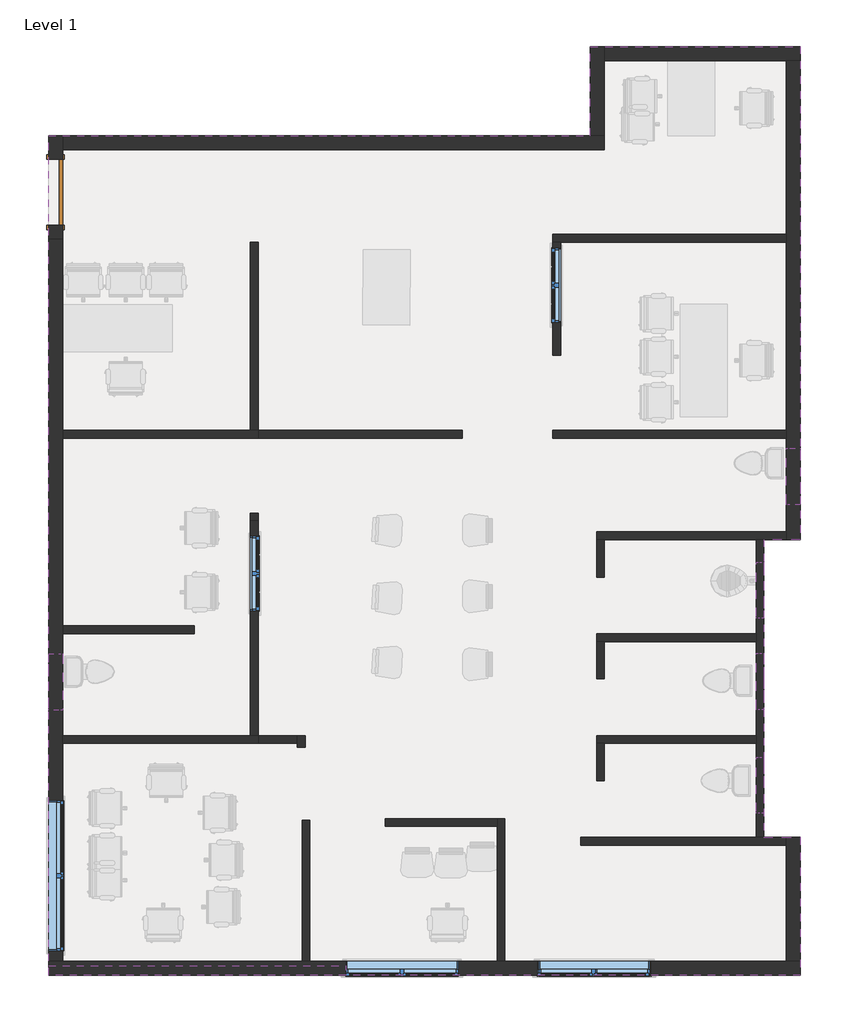
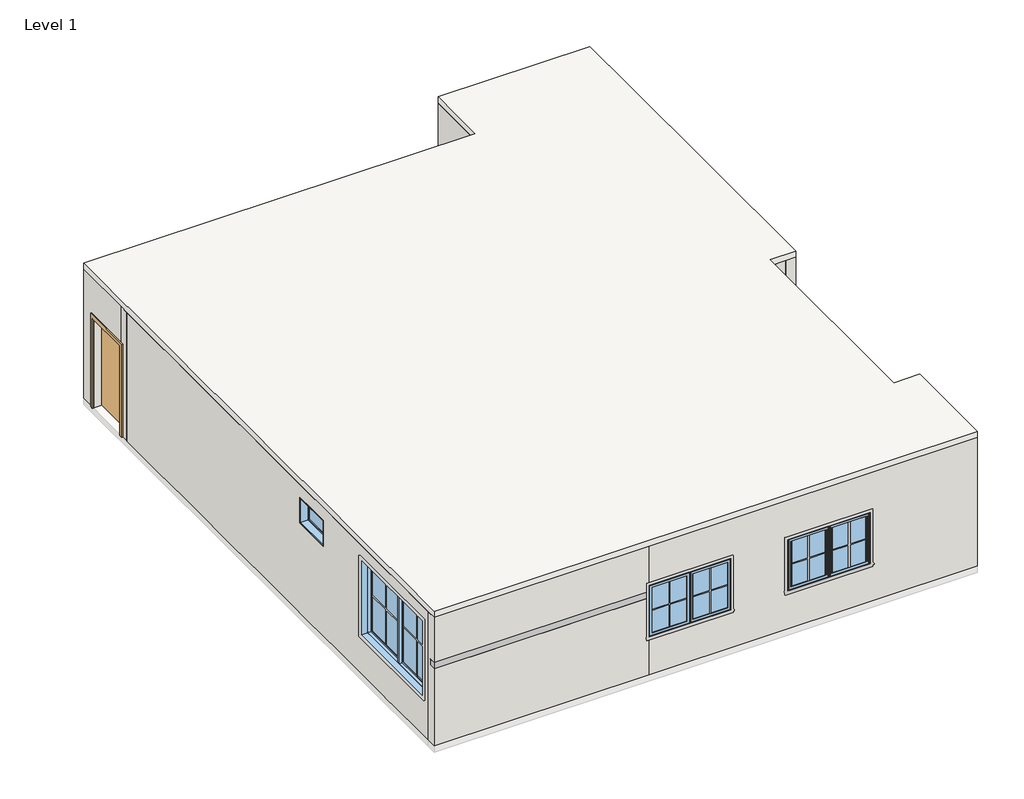
# One storey, part 1 of 2: 34 walls, 12 windows, 1 door, 1 proxy, 1 slab.
"""IFC4 building model written with IfcOpenShell, lengths in millimetres."""

from ifc_helpers import new_model, si_unit, frame, origin, origin_with_axes, place, context, project, spatial, polyline, outline, extrude, faceted_brep, transform, mapped, element, save
from components import door_0848dd25, window_12349545, window_a7c9e031, window_c8489cfa, window_casement_double_4_52a76413, window_casement_double_4_x4_bf2f09a8, window_casement_double_6_x4_44178710, window_casement_double_8_9ae172a2

model = new_model("IFC4")

# Units and contexts
model_context = context("Model", 3, world=origin())
ifc_project = project(units=[si_unit("LENGTHUNIT", "METRE", prefix="MILLI")], contexts=[model_context])

# Site, building, storey
site = spatial("IfcSite", under=ifc_project)
building = spatial("IfcBuilding", under=site)
storey = spatial("IfcBuildingStorey", under=building, Name="Level 1", Elevation=0.0)

# Proxy
placement = place(None, origin())
element("IfcBuildingElementProxy", 1, Name="Reveal", ObjectType="Reveal", at=placement, inside=storey, context=model_context, shape_type="SweptSolid", body=[
    extrude(outline(polyline([(-7315.2, -5486.4), (-7315.2, -5334.0), (-2495.8695713, -5334.0), (-2495.8695713, -5486.4), (-7315.2, -5486.4)])), frame((0.0, 0.0, 1828.8), z_axis=(0.0, 0.0, 1.0), x_axis=(1.0, 0.0, 0.0)), (0.0, 0.0, 1.0), 152.4),
])

# Door
door_shape = door_0848dd25(model_context)
element("IfcDoor", 2, ObjectType="Single-Flush : 3'6\"X7'", at=placement, inside=storey, context=model_context, shape_type="MappedRepresentation", body=[
    mapped(door_shape, transform((-7200.9, 7213.6129621, 0.0), x_axis=(0.0, 1.0, 0.0), y_axis=(-1.0, 0.0, 0.0), z_axis=(0.0, 0.0, 1.0))),
])

# Slab
element("IfcSlab", 3, ObjectType="Generic - 6\"", at=placement, inside=storey, context=model_context, shape_type="SweptSolid", body=[
    extrude(outline(polyline([(1473.2, 8128.0), (1473.2, 9575.8), (4876.8, 9575.8), (4876.8, 8128.0), (4876.8, 1574.8), (4289.425, 1574.8), (4289.425, -3251.2), (4876.8, -3251.2), (4876.8, -5486.4), (-7315.2, -5486.4), (-7315.2, 8128.0), (1473.2, 8128.0)])), frame((0.0, 0.0, 3048.0), z_axis=(0.0, 0.0, 1.0), x_axis=(1.0, 0.0, 0.0)), (0.0, 0.0, 1.0), 152.4),
])

# Walls
element("IfcWall", 4, at=placement, inside=storey, context=model_context, shape_type="Brep", body=[
    faceted_brep([(-7315.2, -5486.4, 0.0), (-2495.8695713, -5486.4, 0.0), (-2495.8695713, -5486.4, 914.4), (-2495.8695713, -5486.4, 1828.8), (-7315.2, -5486.4, 1828.8), (-2495.8695713, -5486.4, 3048.0), (-7315.2, -5486.4, 3048.0), (-7315.2, -5486.4, 1981.2), (-2495.8695713, -5486.4, 1981.2), (-2495.8695713, -5486.4, 2133.6), (-2495.8695713, -5257.8, 0.0), (-3073.4, -5257.8, 0.0), (-3200.4, -5257.8, 0.0), (-7086.6, -5257.8, 0.0), (-7315.2, -5257.8, 0.0), (-7315.2, -5257.8, 3048.0), (-7086.6, -5257.8, 3048.0), (-3200.4, -5257.8, 3048.0), (-3073.4, -5257.8, 3048.0), (-2495.8695713, -5257.8, 3048.0), (-2495.8695713, -5257.8, 2133.6), (-2495.8695713, -5257.8, 914.4), (-2495.8695713, -5334.0, 1981.2), (-2495.8695713, -5334.0, 1828.8), (-7315.2, -5334.0, 1828.8), (-7315.2, -5334.0, 1981.2)], [[[0, 1, 2, 3, 4]], [[5, 6, 7, 8, 9]], [[10, 11, 12, 13, 14, 15, 16, 17, 18, 19, 20, 21]], [[1, 0, 14, 13, 12, 11, 10]], [[10, 21, 20, 19, 5, 9, 8, 22, 23, 3, 2, 1]], [[6, 5, 19, 18, 17, 16, 15]], [[6, 15, 14, 0, 4, 24, 25, 7]], [[25, 22, 8, 7]], [[22, 25, 24, 23]], [[23, 24, 4, 3]]]),
])
element("IfcWall", 5, at=placement, inside=storey, context=model_context, shape_type="SweptSolid", body=[
    extrude(outline(polyline([(-3073.4, -2971.8), (-3073.4, -5257.8), (-3200.4, -5257.8), (-3200.4, -2971.8), (-3073.4, -2971.8)])), origin_with_axes(), (0.0, 0.0, 1.0), 3048.0),
])
element("IfcWall", 6, at=placement, inside=storey, context=model_context, shape_type="SweptSolid", body=[
    extrude(outline(polyline([(-4953.0, 50.8), (-7086.6, 50.8), (-7086.6, 177.8), (-4953.0, 177.8), (-4953.0, 50.8)])), origin_with_axes(), (0.0, 0.0, 1.0), 3048.0),
])
element("IfcWall", 7, ObjectType="3'", at=placement, inside=storey, context=model_context, shape_type="Brep", body=[
    faceted_brep([(4289.425, -3251.2, 0.0), (4289.425, 1574.8, 0.0), (4289.425, 1574.8, 3048.0), (4289.425, -3251.2, 3048.0), (4289.425, -2864.0421459, 2743.2), (4289.425, -1949.6421459, 2743.2), (4289.425, -1949.6421459, 2133.6), (4289.425, -2864.0421459, 2133.6), (4289.425, -266.6798193, 2743.2), (4289.425, -266.6798193, 2133.6), (4289.425, -1181.0798193, 2133.6), (4289.425, -1181.0798193, 2743.2), (4289.425, 299.1205911, 2743.2), (4289.425, 1213.5205911, 2743.2), (4289.425, 1213.5205911, 2133.6), (4289.425, 299.1205911, 2133.6), (4162.425, -3251.2, 0.0), (4162.425, -3251.2, 3048.0), (4162.425, -1727.2, 3048.0), (4162.425, -1600.2, 3048.0), (4162.425, -76.2, 3048.0), (4162.425, 50.8, 3048.0), (4162.425, 1574.8, 3048.0), (4162.425, 1574.8, 0.0), (4162.425, 50.8, 0.0), (4162.425, -76.2, 0.0), (4162.425, -1600.2, 0.0), (4162.425, -1727.2, 0.0), (4162.425, -2864.0421459, 2743.2), (4162.425, -2864.0421459, 2133.6), (4162.425, -1949.6421459, 2133.6), (4162.425, -1949.6421459, 2743.2), (4162.425, -266.6798193, 2743.2), (4162.425, -1181.0798193, 2743.2), (4162.425, -1181.0798193, 2133.6), (4162.425, -266.6798193, 2133.6), (4162.425, 299.1205911, 2743.2), (4162.425, 299.1205911, 2133.6), (4162.425, 1213.5205911, 2133.6), (4162.425, 1213.5205911, 2743.2)], [[[0, 1, 2, 3], [4, 5, 6, 7], [8, 9, 10, 11], [12, 13, 14, 15]], [[16, 17, 18, 19, 20, 21, 22, 23, 24, 25, 26, 27], [28, 29, 30, 31], [32, 33, 34, 35], [36, 37, 38, 39]], [[1, 0, 16, 27, 26, 25, 24, 23]], [[3, 2, 22, 21, 20, 19, 18, 17]], [[0, 3, 17, 16]], [[2, 1, 23, 22]], [[29, 28, 4, 7]], [[30, 29, 7, 6]], [[31, 30, 6, 5]], [[28, 31, 5, 4]], [[9, 8, 32, 35]], [[10, 9, 35, 34]], [[11, 10, 34, 33]], [[8, 11, 33, 32]], [[37, 36, 12, 15]], [[38, 37, 15, 14]], [[39, 38, 14, 13]], [[36, 39, 13, 12]]]),
])
element("IfcWall", 8, ObjectType="WALL11", at=placement, inside=storey, context=model_context, shape_type="Brep", body=[
    faceted_brep([(-2495.8695713, -5486.4, 0.0), (4876.8, -5486.4, 0.0), (4876.8, -5486.4, 3048.0), (-2495.8695713, -5486.4, 3048.0), (-2495.8695713, -5486.4, 2133.6), (-667.0695713, -5486.4, 2133.6), (-667.0695713, -5486.4, 914.4), (-2495.8695713, -5486.4, 914.4), (2463.8, -5486.4, 914.4), (609.6, -5486.4, 914.4), (609.6, -5486.4, 2133.6), (2463.8, -5486.4, 2133.6), (4876.8, -5257.8, 0.0), (4648.2, -5257.8, 0.0), (88.9, -5257.8, 0.0), (-38.1, -5257.8, 0.0), (-2495.8695713, -5257.8, 0.0), (-2495.8695713, -5257.8, 914.4), (-667.0695713, -5257.8, 914.4), (-667.0695713, -5257.8, 2133.6), (-2495.8695713, -5257.8, 2133.6), (-2495.8695713, -5257.8, 3048.0), (-38.1, -5257.8, 3048.0), (88.9, -5257.8, 3048.0), (4648.2, -5257.8, 3048.0), (4876.8, -5257.8, 3048.0), (2463.8, -5257.8, 2133.6), (609.6, -5257.8, 2133.6), (609.6, -5257.8, 914.4), (2463.8, -5257.8, 914.4)], [[[0, 1, 2, 3, 4, 5, 6, 7], [8, 9, 10, 11]], [[12, 13, 14, 15, 16, 17, 18, 19, 20, 21, 22, 23, 24, 25], [26, 27, 28, 29]], [[1, 0, 16, 15, 14, 13, 12]], [[3, 2, 25, 24, 23, 22, 21]], [[3, 21, 20, 4]], [[16, 0, 7, 17]], [[2, 1, 12, 25]], [[5, 19, 18, 6]], [[6, 18, 17, 7]], [[19, 5, 4, 20]], [[28, 27, 10, 9]], [[28, 9, 8, 29]], [[10, 27, 26, 11]], [[29, 8, 11, 26]]]),
])
element("IfcWall", 9, ObjectType="WALL12", at=placement, inside=storey, context=model_context, shape_type="Brep", body=[
    faceted_brep([(4876.8, -5257.8, 0.0), (4876.8, -3251.2, 0.0), (4876.8, -3251.2, 3048.0), (4876.8, -5257.8, 3048.0), (4648.2, -5257.8, 0.0), (4648.2, -5257.8, 3048.0), (4648.2, -3378.2, 3048.0), (4648.2, -3251.2, 3048.0), (4648.2, -3251.2, 0.0), (4648.2, -3378.2, 0.0)], [[[0, 1, 2, 3]], [[4, 5, 6, 7, 8, 9]], [[1, 0, 4, 9, 8]], [[3, 2, 7, 6, 5]], [[0, 3, 5, 4]], [[2, 1, 8, 7]]]),
])
element("IfcWall", 10, ObjectType="WALL13", at=placement, inside=storey, context=model_context, shape_type="Brep", body=[
    faceted_brep([(4648.2, -3251.2, 0.0), (4289.425, -3251.2, 0.0), (4162.425, -3251.2, 0.0), (1320.7323113, -3251.2, 0.0), (1320.7323113, -3251.2, 3048.0), (4162.425, -3251.2, 3048.0), (4289.425, -3251.2, 3048.0), (4648.2, -3251.2, 3048.0), (4648.2, -3378.2, 0.0), (4648.2, -3378.2, 3048.0), (1320.7323113, -3378.2, 3048.0), (1320.7323113, -3378.2, 0.0)], [[[0, 1, 2, 3, 4, 5, 6, 7]], [[8, 9, 10, 11]], [[3, 2, 1, 0, 8, 11]], [[4, 3, 11, 10]], [[7, 6, 5, 4, 10, 9]], [[0, 7, 9, 8]]]),
])
element("IfcWall", 11, ObjectType="WALL16 2", at=placement, inside=storey, context=model_context, shape_type="Brep", body=[
    faceted_brep([(4162.425, -1600.2, 0.0), (1574.8, -1600.2, 0.0), (1574.8, -1600.2, 3048.0), (4162.425, -1600.2, 3048.0), (4162.425, -1727.2, 0.0), (4162.425, -1727.2, 3048.0), (1701.8, -1727.2, 3048.0), (1574.8, -1727.2, 3048.0), (1574.8, -1727.2, 0.0), (1701.8, -1727.2, 0.0)], [[[0, 1, 2, 3]], [[4, 5, 6, 7, 8, 9]], [[1, 0, 4, 9, 8]], [[3, 2, 7, 6, 5]], [[0, 3, 5, 4]], [[2, 1, 8, 7]]]),
])
element("IfcWall", 12, ObjectType="WALL16 2", at=placement, inside=storey, context=model_context, shape_type="SweptSolid", body=[
    extrude(outline(polyline([(1574.8, -2333.2020056), (1574.8, -1727.2), (1701.8, -1727.2), (1701.8, -2333.2020056), (1574.8, -2333.2020056)])), origin_with_axes(), (0.0, 0.0, 1.0), 3048.0),
])
element("IfcWall", 13, ObjectType="WALL17", at=placement, inside=storey, context=model_context, shape_type="Brep", body=[
    faceted_brep([(4162.425, 50.8, 0.0), (1574.8, 50.8, 0.0), (1574.8, 50.8, 3048.0), (4162.425, 50.8, 3048.0), (4162.425, -76.2, 0.0), (4162.425, -76.2, 3048.0), (1701.8, -76.2, 3048.0), (1574.8, -76.2, 3048.0), (1574.8, -76.2, 0.0), (1701.8, -76.2, 0.0)], [[[0, 1, 2, 3]], [[4, 5, 6, 7, 8, 9]], [[1, 0, 4, 9, 8]], [[3, 2, 7, 6, 5]], [[0, 3, 5, 4]], [[2, 1, 8, 7]]]),
])
element("IfcWall", 14, ObjectType="WALL17", at=placement, inside=storey, context=model_context, shape_type="SweptSolid", body=[
    extrude(outline(polyline([(1574.8, -682.1332616), (1574.8, -76.2), (1701.8, -76.2), (1701.8, -682.1332616), (1574.8, -682.1332616)])), origin_with_axes(), (0.0, 0.0, 1.0), 3048.0),
])
element("IfcWall", 15, ObjectType="WALL18", at=placement, inside=storey, context=model_context, shape_type="Brep", body=[
    faceted_brep([(4648.2, 1701.8, 0.0), (1574.8, 1701.8, 0.0), (1574.8, 1701.8, 3048.0), (4648.2, 1701.8, 3048.0), (4648.2, 1574.8, 0.0), (4648.2, 1574.8, 3048.0), (4289.425, 1574.8, 3048.0), (4162.425, 1574.8, 3048.0), (1701.8, 1574.8, 3048.0), (1574.8, 1574.8, 3048.0), (1574.8, 1574.8, 0.0), (1701.8, 1574.8, 0.0), (4162.425, 1574.8, 0.0), (4289.425, 1574.8, 0.0)], [[[0, 1, 2, 3]], [[4, 5, 6, 7, 8, 9, 10, 11, 12, 13]], [[1, 0, 4, 13, 12, 11, 10]], [[3, 2, 9, 8, 7, 6, 5]], [[0, 3, 5, 4]], [[2, 1, 10, 9]]]),
])
element("IfcWall", 16, ObjectType="WALL18", at=placement, inside=storey, context=model_context, shape_type="SweptSolid", body=[
    extrude(outline(polyline([(1574.8, 965.114599), (1574.8, 1574.8), (1701.8, 1574.8), (1701.8, 965.114599), (1574.8, 965.114599)])), origin_with_axes(), (0.0, 0.0, 1.0), 3048.0),
])
element("IfcWall", 17, ObjectType="WALL19", at=placement, inside=storey, context=model_context, shape_type="SweptSolid", body=[
    extrude(outline(polyline([(863.6, 3352.8), (4648.2, 3352.8), (4648.2, 3225.8), (863.6, 3225.8), (863.6, 3352.8)])), origin_with_axes(), (0.0, 0.0, 1.0), 3048.0),
])
element("IfcWall", 18, ObjectType="WALL20", at=placement, inside=storey, context=model_context, shape_type="Brep", body=[
    faceted_brep([(4648.2, 6527.8, 0.0), (863.6, 6527.8, 0.0), (863.6, 6527.8, 3048.0), (4648.2, 6527.8, 3048.0), (4648.2, 6400.8, 0.0), (4648.2, 6400.8, 3048.0), (990.6, 6400.8, 3048.0), (863.6, 6400.8, 3048.0), (863.6, 6400.8, 0.0), (990.6, 6400.8, 0.0)], [[[0, 1, 2, 3]], [[4, 5, 6, 7, 8, 9]], [[1, 0, 4, 9, 8]], [[3, 2, 7, 6, 5]], [[0, 3, 5, 4]], [[2, 1, 8, 7]]]),
])
element("IfcWall", 19, ObjectType="WALL20", at=placement, inside=storey, context=model_context, shape_type="SweptSolid", body=[
    extrude(outline(polyline([(6400.8, 0.0), (4571.3294041, 0.0), (4571.3294041, 3048.0), (6400.8, 3048.0), (6400.8, 0.0)]), holes=[polyline([(6311.9, 2743.2), (5092.7, 2743.2), (5092.7, 914.4), (6311.9, 914.4), (6311.9, 2743.2)])]), frame((863.6, 0.0, 0.0), z_axis=(1.0, 0.0, 0.0), x_axis=(0.0, 1.0, 0.0)), (0.0, 0.0, 1.0), 127.0),
])
element("IfcWall", 20, ObjectType="WALL21", at=placement, inside=storey, context=model_context, shape_type="Brep", body=[
    faceted_brep([(-7086.6, 3225.8, 0.0), (-3911.6, 3225.8, 0.0), (-3911.6, 3225.8, 3048.0), (-7086.6, 3225.8, 3048.0), (-7086.6, 3352.8, 0.0), (-7086.6, 3352.8, 3048.0), (-4038.6, 3352.8, 3048.0), (-3911.6, 3352.8, 3048.0), (-3911.6, 3352.8, 0.0), (-4038.6, 3352.8, 0.0)], [[[0, 1, 2, 3]], [[4, 5, 6, 7, 8, 9]], [[1, 0, 4, 9, 8]], [[3, 2, 7, 6, 5]], [[0, 3, 5, 4]], [[2, 1, 8, 7]]]),
])
element("IfcWall", 21, ObjectType="WALL21", at=placement, inside=storey, context=model_context, shape_type="SweptSolid", body=[
    extrude(outline(polyline([(-3911.6, 6400.8), (-3911.6, 3352.8), (-4038.6, 3352.8), (-4038.6, 6400.8), (-3911.6, 6400.8)])), origin_with_axes(), (0.0, 0.0, 1.0), 3048.0),
])
element("IfcWall", 22, ObjectType="WALL23 2", at=placement, inside=storey, context=model_context, shape_type="Brep", body=[
    faceted_brep([(-7086.6, -1727.2, 0.0), (-3911.6, -1727.2, 0.0), (-3911.6, -1727.2, 3048.0), (-7086.6, -1727.2, 3048.0), (-7086.6, -1600.2, 0.0), (-7086.6, -1600.2, 3048.0), (-4038.6, -1600.2, 3048.0), (-3911.6, -1600.2, 3048.0), (-3911.6, -1600.2, 0.0), (-4038.6, -1600.2, 0.0)], [[[0, 1, 2, 3]], [[4, 5, 6, 7, 8, 9]], [[1, 0, 4, 9, 8]], [[3, 2, 7, 6, 5]], [[0, 3, 5, 4]], [[2, 1, 8, 7]]]),
])
element("IfcWall", 23, ObjectType="WALL23 2", at=placement, inside=storey, context=model_context, shape_type="SweptSolid", body=[
    extrude(outline(polyline([(-1600.2, 0.0), (-1600.2, 3048.0), (1880.1111463, 3048.0), (1880.1111463, 0.0), (-1600.2, 0.0)]), holes=[polyline([(419.6111463, 2743.2), (419.6111463, 914.4), (1638.8111463, 914.4), (1638.8111463, 2743.2), (419.6111463, 2743.2)])]), frame((-4038.6, 0.0, 0.0), z_axis=(1.0, 0.0, 0.0), x_axis=(0.0, 1.0, 0.0)), (0.0, 0.0, 1.0), 127.0),
])
element("IfcWall", 24, ObjectType="WALL23 2", at=placement, inside=storey, context=model_context, shape_type="SweptSolid", body=[
    extrude(outline(polyline([(-3911.6, 1880.1111463), (-4038.6, 1880.1111463), (-4038.6, 2007.1111463), (-3911.6, 2007.1111463), (-3911.6, 1880.1111463)])), origin_with_axes(), (0.0, 0.0, 1.0), 3048.0),
])
element("IfcWall", 25, ObjectType="WALL23 2", at=placement, inside=storey, context=model_context, shape_type="SweptSolid", body=[
    extrude(outline(polyline([(1880.1111463, 0.0), (-1600.2, 0.0), (-1600.2, 3048.0), (1880.1111463, 3048.0), (1880.1111463, 0.0)]), holes=[polyline([(419.6111463, 2743.2), (419.6111463, 914.4), (1638.8111463, 914.4), (1638.8111463, 2743.2), (419.6111463, 2743.2)])]), frame((-4038.6, 0.0, 0.0), z_axis=(1.0, 0.0, 0.0), x_axis=(0.0, 1.0, 0.0)), (0.0, 0.0, 1.0), 127.0),
])
element("IfcWall", 26, ObjectType="WALL23 2", at=placement, inside=storey, context=model_context, shape_type="Brep", body=[
    faceted_brep([(-3276.6, -1600.2, 0.0), (-3276.6, -1727.2, 0.0), (-3276.6, -1790.7, 0.0), (-3276.6, -1790.7, 3048.0), (-3276.6, -1727.2, 3048.0), (-3276.6, -1600.2, 3048.0), (-3149.6, -1600.2, 0.0), (-3149.6, -1600.2, 3048.0), (-3149.6, -1790.7, 3048.0), (-3149.6, -1790.7, 0.0)], [[[0, 1, 2, 3, 4, 5]], [[6, 7, 8, 9]], [[2, 1, 0, 6, 9]], [[3, 2, 9, 8]], [[5, 4, 3, 8, 7]], [[0, 5, 7, 6]]]),
])
element("IfcWall", 27, ObjectType="WALL24", at=placement, inside=storey, context=model_context, shape_type="SweptSolid", body=[
    extrude(outline(polyline([(-3276.6, -1727.2), (-3911.6, -1727.2), (-3911.6, -1600.2), (-3276.6, -1600.2), (-3276.6, -1727.2)])), origin_with_axes(), (0.0, 0.0, 1.0), 3048.0),
])
element("IfcWall", 28, ObjectType="WALL26", at=placement, inside=storey, context=model_context, shape_type="SweptSolid", body=[
    extrude(outline(polyline([(-601.4207418, 3225.8), (-3911.6, 3225.8), (-3911.6, 3352.8), (-601.4207418, 3352.8), (-601.4207418, 3225.8)])), origin_with_axes(), (0.0, 0.0, 1.0), 3048.0),
])
element("IfcWall", 29, ObjectType="WALL28", at=placement, inside=storey, context=model_context, shape_type="Brep", body=[
    faceted_brep([(88.9, -5257.8, 0.0), (88.9, -2946.3624245, 0.0), (88.9, -2946.3624245, 3048.0), (88.9, -5257.8, 3048.0), (-38.1, -5257.8, 0.0), (-38.1, -5257.8, 3048.0), (-38.1, -3073.3624245, 3048.0), (-38.1, -2946.3624245, 3048.0), (-38.1, -2946.3624245, 0.0), (-38.1, -3073.3624245, 0.0)], [[[0, 1, 2, 3]], [[4, 5, 6, 7, 8, 9]], [[1, 0, 4, 9, 8]], [[3, 2, 7, 6, 5]], [[0, 3, 5, 4]], [[2, 1, 8, 7]]]),
])
element("IfcWall", 30, ObjectType="WALL29", at=placement, inside=storey, context=model_context, shape_type="SweptSolid", body=[
    extrude(outline(polyline([(-1854.625458, -2946.3624245), (-38.1, -2946.3624245), (-38.1, -3073.3624245), (-1854.625458, -3073.3624245), (-1854.625458, -2946.3624245)])), origin_with_axes(), (0.0, 0.0, 1.0), 3048.0),
])
element("IfcWall", 31, ObjectType="WALL6", at=placement, inside=storey, context=model_context, shape_type="Brep", body=[
    faceted_brep([(-7086.6, 8128.0, 3048.0), (-7086.6, 7899.4, 3048.0), (-7086.6, 6680.2210262, 3048.0), (-7086.6, 6680.2210262, 2133.6), (-7086.6, 7747.0129621, 2133.6), (-7086.6, 7747.0129621, 0.0), (-7086.6, 7899.4, 0.0), (-7086.6, 8128.0, 0.0), (-7315.2, 6680.2210262, 3048.0), (-7315.2, 8128.0, 3048.0), (-7315.2, 8128.0, 0.0), (-7315.2, 7747.0129621, 0.0), (-7315.2, 7747.0129621, 2133.6), (-7315.2, 6680.2210262, 2133.6)], [[[0, 1, 2, 3, 4, 5, 6, 7]], [[8, 9, 10, 11, 12, 13]], [[10, 7, 6, 5, 11]], [[2, 1, 0, 9, 8]], [[0, 7, 10, 9]], [[2, 8, 13, 3]], [[4, 12, 11, 5]], [[12, 4, 3, 13]]]),
])
element("IfcWall", 32, ObjectType="WALL6", at=placement, inside=storey, context=model_context, shape_type="Brep", body=[
    faceted_brep([(-7086.6, 7899.4, 0.0), (1701.8, 7899.4, 0.0), (1701.8, 7899.4, 3048.0), (-7086.6, 7899.4, 3048.0), (-7086.6, 8128.0, 0.0), (-7086.6, 8128.0, 3048.0), (1473.2, 8128.0, 3048.0), (1701.8, 8128.0, 3048.0), (1701.8, 8128.0, 0.0), (1473.2, 8128.0, 0.0)], [[[0, 1, 2, 3]], [[4, 5, 6, 7, 8, 9]], [[1, 0, 4, 9, 8]], [[3, 2, 7, 6, 5]], [[0, 3, 5, 4]], [[2, 1, 8, 7]]]),
])
element("IfcWall", 33, ObjectType="WALL6", at=placement, inside=storey, context=model_context, shape_type="Brep", body=[
    faceted_brep([(1701.8, 8128.0, 0.0), (1701.8, 9347.2, 0.0), (1701.8, 9575.8, 0.0), (1701.8, 9575.8, 3048.0), (1701.8, 9347.2, 3048.0), (1701.8, 8128.0, 3048.0), (1473.2, 8128.0, 0.0), (1473.2, 8128.0, 3048.0), (1473.2, 9575.8, 3048.0), (1473.2, 9575.8, 0.0)], [[[0, 1, 2, 3, 4, 5]], [[6, 7, 8, 9]], [[2, 1, 0, 6, 9]], [[5, 4, 3, 8, 7]], [[0, 5, 7, 6]], [[3, 2, 9, 8]]]),
])
element("IfcWall", 34, ObjectType="WALL8", at=placement, inside=storey, context=model_context, shape_type="Brep", body=[
    faceted_brep([(1701.8, 9347.2, 0.0), (4648.2, 9347.2, 0.0), (4876.8, 9347.2, 0.0), (4876.8, 9347.2, 3048.0), (4648.2, 9347.2, 3048.0), (1701.8, 9347.2, 3048.0), (1701.8, 9575.8, 0.0), (1701.8, 9575.8, 3048.0), (4876.8, 9575.8, 3048.0), (4876.8, 9575.8, 0.0)], [[[0, 1, 2, 3, 4, 5]], [[6, 7, 8, 9]], [[2, 1, 0, 6, 9]], [[5, 4, 3, 8, 7]], [[0, 5, 7, 6]], [[3, 2, 9, 8]]]),
])
element("IfcWall", 35, ObjectType="WALL8", at=placement, inside=storey, context=model_context, shape_type="Brep", body=[
    faceted_brep([(4648.2, 9347.2, 0.0), (4648.2, 6527.8, 0.0), (4648.2, 6400.8, 0.0), (4648.2, 3352.8, 0.0), (4648.2, 3225.8, 0.0), (4648.2, 1701.8, 0.0), (4648.2, 1574.8, 0.0), (4648.2, 1574.8, 3048.0), (4648.2, 1701.8, 3048.0), (4648.2, 3225.8, 3048.0), (4648.2, 3352.8, 3048.0), (4648.2, 6400.8, 3048.0), (4648.2, 6527.8, 3048.0), (4648.2, 9347.2, 3048.0), (4648.2, 3060.7, 2743.2), (4648.2, 2146.3, 2743.2), (4648.2, 2146.3, 2133.6), (4648.2, 3060.7, 2133.6), (4876.8, 9347.2, 0.0), (4876.8, 9347.2, 3048.0), (4876.8, 1574.8, 3048.0), (4876.8, 1574.8, 0.0), (4876.8, 3060.7, 2743.2), (4876.8, 3060.7, 2133.6), (4876.8, 2146.3, 2133.6), (4876.8, 2146.3, 2743.2)], [[[0, 1, 2, 3, 4, 5, 6, 7, 8, 9, 10, 11, 12, 13], [14, 15, 16, 17]], [[18, 19, 20, 21], [22, 23, 24, 25]], [[6, 5, 4, 3, 2, 1, 0, 18, 21]], [[13, 12, 11, 10, 9, 8, 7, 20, 19]], [[0, 13, 19, 18]], [[7, 6, 21, 20]], [[23, 22, 14, 17]], [[24, 23, 17, 16]], [[25, 24, 16, 15]], [[22, 25, 15, 14]]]),
])
element("IfcWall", 36, ObjectType="WALL9", at=placement, inside=storey, context=model_context, shape_type="Brep", body=[
    faceted_brep([(-7315.2, 6451.6210262, 0.0), (-7086.6, 6451.6210262, 0.0), (-7086.6, 6451.6210262, 3048.0), (-7315.2, 6451.6210262, 3048.0), (-7315.2, 6680.2210262, 0.0), (-7315.2, 6680.2210262, 2133.6), (-7315.2, 6680.2210262, 3048.0), (-7086.6, 6680.2210262, 3048.0), (-7086.6, 6680.2210262, 2133.6), (-7086.6, 6680.2210262, 0.0)], [[[0, 1, 2, 3]], [[4, 5, 6, 7, 8, 9]], [[1, 0, 4, 9]], [[3, 2, 7, 6]], [[0, 3, 6, 5, 4]], [[2, 1, 9, 8, 7]]]),
])
element("IfcWall", 37, ObjectType="WALL9", at=placement, inside=storey, context=model_context, shape_type="Brep", body=[
    faceted_brep([(-7315.2, 6451.6210262, 0.0), (-7315.2, -5257.8, 0.0), (-7315.2, -5257.8, 3048.0), (-7315.2, 6451.6210262, 3048.0), (-7315.2, -273.05, 2743.2), (-7315.2, -1187.45, 2743.2), (-7315.2, -1187.45, 2133.6), (-7315.2, -273.05, 2133.6), (-7315.2, -5092.7, 2743.2), (-7315.2, -5092.7, 914.4), (-7315.2, -2654.3, 914.4), (-7315.2, -2654.3, 2743.2), (-7086.6, -5257.8, 0.0), (-7086.6, -1727.2, 0.0), (-7086.6, -1600.2, 0.0), (-7086.6, 50.8, 0.0), (-7086.6, 177.8, 0.0), (-7086.6, 3225.8, 0.0), (-7086.6, 3352.8, 0.0), (-7086.6, 6451.6210262, 0.0), (-7086.6, 6451.6210262, 3048.0), (-7086.6, 3352.8, 3048.0), (-7086.6, 3225.8, 3048.0), (-7086.6, 177.8, 3048.0), (-7086.6, 50.8, 3048.0), (-7086.6, -1600.2, 3048.0), (-7086.6, -1727.2, 3048.0), (-7086.6, -5257.8, 3048.0), (-7086.6, -273.05, 2743.2), (-7086.6, -273.05, 2133.6), (-7086.6, -1187.45, 2133.6), (-7086.6, -1187.45, 2743.2), (-7086.6, -5092.7, 2743.2), (-7086.6, -2654.3, 2743.2), (-7086.6, -2654.3, 914.4), (-7086.6, -5092.7, 914.4)], [[[0, 1, 2, 3], [4, 5, 6, 7], [8, 9, 10, 11]], [[12, 13, 14, 15, 16, 17, 18, 19, 20, 21, 22, 23, 24, 25, 26, 27], [28, 29, 30, 31], [32, 33, 34, 35]], [[1, 0, 19, 18, 17, 16, 15, 14, 13, 12]], [[3, 2, 27, 26, 25, 24, 23, 22, 21, 20]], [[2, 1, 12, 27]], [[0, 3, 20, 19]], [[29, 28, 4, 7]], [[30, 29, 7, 6]], [[31, 30, 6, 5]], [[28, 31, 5, 4]], [[9, 8, 32, 35]], [[10, 9, 35, 34]], [[11, 10, 34, 33]], [[8, 11, 33, 32]]]),
])

# Windows
window_shape = window_12349545(model_context)
element("IfcWindow", 38, ObjectType="Fixed : 36\" x 24\"", at=placement, inside=storey, context=model_context, shape_type="MappedRepresentation", body=[
    mapped(window_shape, transform((4225.925, -2444.9421459, 0.0), x_axis=(0.0, -1.0, 0.0), y_axis=(1.0, 0.0, 0.0), z_axis=(0.0, 0.0, 1.0))),
])
element("IfcWindow", 39, ObjectType="Fixed : 36\" x 24\"", at=placement, inside=storey, context=model_context, shape_type="MappedRepresentation", body=[
    mapped(window_shape, transform((4225.925, -685.7798193, 0.0), x_axis=(0.0, 1.0, 0.0), y_axis=(-1.0, 0.0, 0.0), z_axis=(0.0, 0.0, 1.0))),
])
element("IfcWindow", 40, ObjectType="Fixed : 36\" x 24\"", at=placement, inside=storey, context=model_context, shape_type="MappedRepresentation", body=[
    mapped(window_shape, transform((4225.925, 718.2205911, 0.0), x_axis=(0.0, -1.0, 0.0), y_axis=(1.0, 0.0, 0.0), z_axis=(0.0, 0.0, 1.0))),
])
window_2_shape = window_a7c9e031(model_context)
element("IfcWindow", 41, ObjectType="Fixed : 36\" x 24\"", at=placement, inside=storey, context=model_context, shape_type="MappedRepresentation", body=[
    mapped(window_2_shape, transform((4762.5, 2641.6, 0.0), x_axis=(0.0, 1.0, 0.0), y_axis=(-1.0, 0.0, 0.0), z_axis=(0.0, 0.0, 1.0))),
])
window_3_shape = window_c8489cfa(model_context)
element("IfcWindow", 42, ObjectType="Fixed : 36\" x 24\"", at=placement, inside=storey, context=model_context, shape_type="MappedRepresentation", body=[
    mapped(window_3_shape, transform((-7200.9, -692.15, 0.0), x_axis=(0.0, 1.0, 0.0), y_axis=(-1.0, 0.0, 0.0), z_axis=(0.0, 0.0, 1.0))),
])
window_casement_double_4_shape = window_casement_double_4_52a76413(model_context)
element("IfcWindow", 43, ObjectType="Window-Casement-Double : 4'", at=placement, inside=storey, context=model_context, shape_type="MappedRepresentation", body=[
    mapped(window_casement_double_4_shape, transform((-3975.1, 1029.2111463, 0.0), x_axis=(0.0, -1.0, 0.0), y_axis=(1.0, 0.0, 0.0), z_axis=(0.0, 0.0, 1.0))),
])
element("IfcWindow", 44, ObjectType="Window-Casement-Double : 4'", at=placement, inside=storey, context=model_context, shape_type="MappedRepresentation", body=[
    mapped(window_casement_double_4_shape, transform((-3975.1, 1029.2111463, 0.0), x_axis=(0.0, -1.0, 0.0), y_axis=(1.0, 0.0, 0.0), z_axis=(0.0, 0.0, 1.0))),
])
element("IfcWindow", 45, ObjectType="Window-Casement-Double : 4'", at=placement, inside=storey, context=model_context, shape_type="MappedRepresentation", body=[
    mapped(window_casement_double_4_shape, transform((927.1, 5702.3, 0.0), x_axis=(0.0, 1.0, 0.0), y_axis=(-1.0, 0.0, 0.0), z_axis=(0.0, 0.0, 1.0))),
])
window_casement_double_4_x4_shape = window_casement_double_4_x4_bf2f09a8(model_context)
element("IfcWindow", 46, ObjectType="Window-Casement-Double : 4'X4'", at=placement, inside=storey, context=model_context, shape_type="MappedRepresentation", body=[
    mapped(window_casement_double_4_x4_shape, transform((1524.0, -5372.1, 0.0), x_axis=(-1.0, 0.0, 0.0), y_axis=(0.0, -1.0, 0.0), z_axis=(0.0, 0.0, 1.0))),
])
element("IfcWindow", 47, ObjectType="Window-Casement-Double : 4'X4'", at=placement, inside=storey, context=model_context, shape_type="MappedRepresentation", body=[
    mapped(window_casement_double_4_x4_shape, transform((1549.4, -5372.1, 0.0), x_axis=(-1.0, 0.0, 0.0), y_axis=(0.0, -1.0, 0.0), z_axis=(0.0, 0.0, 1.0))),
])
window_casement_double_6_x4_shape = window_casement_double_6_x4_44178710(model_context)
element("IfcWindow", 48, ObjectType="Window-Casement-Double : 6'X4'", at=placement, inside=storey, context=model_context, shape_type="MappedRepresentation", body=[
    mapped(window_casement_double_6_x4_shape, transform((-1581.4695713, -5372.1, 0.0), x_axis=(1.0, 0.0, 0.0), y_axis=(0.0, 1.0, 0.0), z_axis=(0.0, 0.0, 1.0))),
])
window_casement_double_8_shape = window_casement_double_8_9ae172a2(model_context)
element("IfcWindow", 49, ObjectType="Window-Casement-Double : 8'", at=placement, inside=storey, context=model_context, shape_type="MappedRepresentation", body=[
    mapped(window_casement_double_8_shape, transform((-7200.9, -3873.5, 0.0), x_axis=(0.0, -1.0, 0.0), y_axis=(1.0, 0.0, 0.0), z_axis=(0.0, 0.0, 1.0))),
])

save(model, "model.ifc")

# Revit data of these elements
# Type "Single-Flush : 3'6\"X7'"
#   Type Mark = "8"
#   Construction Type Id = "MDOOR"
#   Assembly Code = "C1020"
#   Analytic Construction = "Metal"
#   Thickness = 0' - 2"
#   Heat Transfer Coefficient (U) = 0.651978 BTU/(h·ft²·°F)
#   Height = 7' - 0"
#   Trim Projection Ext = 0' - 1"
#   Trim Projection Int = 0' - 1"
#   Trim Width = 0' - 3"
#   Width = 3' - 6"
#   Define Thermal Properties by = 1
#   Door Material = Door - Panel
#   Frame Material = Door - Frame
#   Visual Light Transmittance = 0
#   Solar Heat Gain Coefficient = 0
#   Function = (empty or 0)
#   Wall Closure = (empty or 0)
# Type "Generic - 6\""
#   Assembly Code = "B1010"
#   Function = 0
#   Layers, outside or top first: 0' - 6" no material (function 1)
# Type
#   Assembly Code = "B2010"
#   Layers, outside or top first: 0' - 9" no material (function 1)
# Type
#   Assembly Code = "B2010"
#   Layers, outside or top first: 0' - 5" no material (function 1)
# Type
#   Assembly Code = "B2010"
#   Layers, outside or top first: 0' - 5" no material (function 1)
# Type "3'"
#   Assembly Code = "B2010"
#   Layers, outside or top first: 0' - 5" no material (function 1)
# Type "WALL11"
#   Assembly Code = "B2010"
#   Layers, outside or top first: 0' - 9" no material (function 1)
# Type "WALL12"
#   Assembly Code = "B2010"
#   Layers, outside or top first: 0' - 9" no material (function 1)
# Type "WALL13"
#   Assembly Code = "B2010"
#   Layers, outside or top first: 0' - 5" no material (function 1)
# Type "WALL16 2"
#   Assembly Code = "B2010"
#   Layers, outside or top first: 0' - 5" no material (function 1)
# Type "WALL17"
#   Assembly Code = "B2010"
#   Layers, outside or top first: 0' - 5" no material (function 1)
# Type "WALL18"
#   Assembly Code = "B2010"
#   Layers, outside or top first: 0' - 5" no material (function 1)
# Type "WALL19"
#   Assembly Code = "B2010"
#   Layers, outside or top first: 0' - 5" no material (function 1)
# Type "WALL20"
#   Assembly Code = "B2010"
#   Layers, outside or top first: 0' - 5" no material (function 1)
# Type "WALL21"
#   Assembly Code = "B2010"
#   Layers, outside or top first: 0' - 5" no material (function 1)
# Type "WALL23 2"
#   Assembly Code = "B2010"
#   Layers, outside or top first: 0' - 5" no material (function 1)
# Type "WALL24"
#   Assembly Code = "B2010"
#   Layers, outside or top first: 0' - 5" no material (function 1)
# Type "WALL26"
#   Assembly Code = "B2010"
#   Layers, outside or top first: 0' - 5" no material (function 1)
# Type "WALL28"
#   Assembly Code = "B2010"
#   Layers, outside or top first: 0' - 5" no material (function 1)
# Type "WALL29"
#   Assembly Code = "B2010"
#   Layers, outside or top first: 0' - 5" no material (function 1)
# Type "WALL6"
#   Assembly Code = "B2010"
#   Layers, outside or top first: 0' - 9" no material (function 1)
# Type "WALL8"
#   Assembly Code = "B2010"
#   Layers, outside or top first: 0' - 9" no material (function 1)
# Type "WALL9"
#   Assembly Code = "B2010"
#   Layers, outside or top first: 0' - 9" no material (function 1)
# Type "Fixed : 36\" x 24\""
#   Type Mark = "8"
#   Construction Type Id = "GSP4R"
#   Assembly Code = "B2020100"
#   Analytic Construction = "1/8 in Pilkington single glazing"
#   Visual Light Transmittance = 0.9
#   Solar Heat Gain Coefficient = 0.78
#   Heat Transfer Coefficient (U) = 0.6496 BTU/(h·ft²·°F)
#   Height = 2' - 0"
#   Default Sill Height = 7' - 0"
#   Width = 3' - 0"
#   Window Inset = 0' - 0 3/4"
#   Define Thermal Properties by = 1
#   Define Thermal Properties by = 1
#   Glass Pane Material = Glass
#   Sash Material = Sash
#   Wall Closure = (empty or 0)
# Type "Window-Casement-Double : 4'"
#   Type Mark = "28"
#   Fire Rating = "0.5h"
#   Assembly Code = "B2020100"
#   Analytic Construction = "Double glazing - domestic"
#   Frame Extension [instance default] = 0' - 0 1/4"
#   Window Inset [instance default] = 0' - 0"
#   Wall Thickness [instance default] = 0' - 6"
#   Interior Wall Closure [instance default] = 0' - 2 1/4"
#   Half Width = 2' - 0"
#   Visual Light Transmittance = 0.81
#   Thermal Resistance (R) = 1.8146 (h·ft²·°F)/BTU
#   Solar Heat Gain Coefficient = 0.76
#   Rough Width = 4' - 0 1/2"
#   Rough Height = 6' - 0 1/2"
#   Height = 6' - 0"
#   Heat Transfer Coefficient (U) = 0.5511 BTU/(h·ft²·°F)
#   Exterior Wall Closure [instance default] = 0' - 1 1/4"
#   Extension Jamb [instance default] = 0' - 2 1/4"
#   Default Sill Height = 3' - 0"
#   Width = 4' - 0"
#   Muntin Visibility = yes
#   Interior Trim Visibility [instance default] = yes
#   Exterior Trim Visibility [instance default] = yes
#   Extension Jamb Visibility [instance default] = yes
#   Interior Trim Material = Wood - Stained
#   Muntin Pattern = Muntin Pattern_2x2 : Muntin Pattern_2x2
#   Interior Trim = Trim-Window-Interior-Flat : Picture Frame
#   Interior Frame Material = Wood - Stained
#   Glass Panel Material = Glass
#   Exterior Trim Material = Clad - White
#   Exterior Trim = Trim-Window-Exterior-Flat : with Sill
#   Exterior Frame Material = Clad - White
#   Wall Closure = (empty or 0)
# Type "Window-Casement-Double : 4'X4'"
#   Type Mark = "19"
#   Fire Rating = "0.5h"
#   Assembly Code = "B2020100"
#   Analytic Construction = "Double glazing - domestic"
#   Frame Extension [instance default] = 0' - 0 1/4"
#   Window Inset [instance default] = 0' - 0"
#   Wall Thickness [instance default] = 0' - 6"
#   Interior Wall Closure [instance default] = 0' - 2 1/4"
#   Half Width = 3' - 0"
#   Visual Light Transmittance = 0.81
#   Thermal Resistance (R) = 1.8146 (h·ft²·°F)/BTU
#   Solar Heat Gain Coefficient = 0.76
#   Rough Width = 6' - 0 1/2"
#   Rough Height = 4' - 0 1/2"
#   Height = 4' - 0"
#   Heat Transfer Coefficient (U) = 0.5511 BTU/(h·ft²·°F)
#   Exterior Wall Closure [instance default] = 0' - 1 1/4"
#   Extension Jamb [instance default] = 0' - 2 1/4"
#   Default Sill Height = 3' - 0"
#   Width = 6' - 0"
#   Muntin Visibility = yes
#   Interior Trim Visibility [instance default] = yes
#   Exterior Trim Visibility [instance default] = yes
#   Extension Jamb Visibility [instance default] = yes
#   Interior Trim Material = Wood - Stained
#   Muntin Pattern = Muntin Pattern_2x2 : Muntin Pattern_2x2
#   Interior Trim = Trim-Window-Interior-Flat : Picture Frame
#   Interior Frame Material = Wood - Stained
#   Glass Panel Material = Glass
#   Exterior Trim Material = Clad - White
#   Exterior Trim = Trim-Window-Exterior-Flat : with Sill
#   Exterior Frame Material = Clad - White
#   Wall Closure = (empty or 0)
# Type "Window-Casement-Double : 6'X4'"
#   Type Mark = "18"
#   Fire Rating = "0.5h"
#   Assembly Code = "B2020100"
#   Analytic Construction = "Double glazing - domestic"
#   Frame Extension [instance default] = 0' - 0 1/4"
#   Window Inset [instance default] = 0' - 0"
#   Wall Thickness [instance default] = 0' - 6"
#   Interior Wall Closure [instance default] = 0' - 2 1/4"
#   Half Width = 3' - 0"
#   Visual Light Transmittance = 0.81
#   Thermal Resistance (R) = 1.8146 (h·ft²·°F)/BTU
#   Solar Heat Gain Coefficient = 0.76
#   Rough Width = 6' - 0 1/2"
#   Rough Height = 4' - 0 1/2"
#   Height = 4' - 0"
#   Heat Transfer Coefficient (U) = 0.5511 BTU/(h·ft²·°F)
#   Exterior Wall Closure [instance default] = 0' - 1 1/4"
#   Extension Jamb [instance default] = 0' - 2 1/4"
#   Default Sill Height = 3' - 0"
#   Width = 6' - 0"
#   Muntin Visibility = yes
#   Interior Trim Visibility [instance default] = yes
#   Exterior Trim Visibility [instance default] = yes
#   Extension Jamb Visibility [instance default] = yes
#   Interior Trim Material = Wood - Stained
#   Muntin Pattern = Muntin Pattern_2x2 : Muntin Pattern_2x2
#   Interior Trim = Trim-Window-Interior-Flat : Picture Frame
#   Interior Frame Material = Wood - Stained
#   Glass Panel Material = Glass
#   Exterior Trim Material = Clad - White
#   Exterior Trim = Trim-Window-Exterior-Flat : with Sill
#   Exterior Frame Material = Clad - White
#   Wall Closure = (empty or 0)
# Type "Window-Casement-Double : 8'"
#   Type Mark = "27"
#   Fire Rating = "0.5h"
#   Assembly Code = "B2020100"
#   Analytic Construction = "Double glazing - domestic"
#   Frame Extension [instance default] = 0' - 0 1/4"
#   Window Inset [instance default] = 0' - 0"
#   Wall Thickness [instance default] = 0' - 6"
#   Interior Wall Closure [instance default] = 0' - 2 1/4"
#   Half Width = 4' - 0"
#   Visual Light Transmittance = 0.81
#   Thermal Resistance (R) = 1.8146 (h·ft²·°F)/BTU
#   Solar Heat Gain Coefficient = 0.76
#   Rough Width = 8' - 0 1/2"
#   Rough Height = 6' - 0 1/2"
#   Height = 6' - 0"
#   Heat Transfer Coefficient (U) = 0.5511 BTU/(h·ft²·°F)
#   Exterior Wall Closure [instance default] = 0' - 1 1/4"
#   Extension Jamb [instance default] = 0' - 2 1/4"
#   Default Sill Height = 3' - 0"
#   Width = 8' - 0"
#   Muntin Visibility = yes
#   Interior Trim Visibility [instance default] = yes
#   Exterior Trim Visibility [instance default] = yes
#   Extension Jamb Visibility [instance default] = yes
#   Interior Trim Material = Wood - Stained
#   Muntin Pattern = Muntin Pattern_2x2 : Muntin Pattern_2x2
#   Interior Trim = Trim-Window-Interior-Flat : Picture Frame
#   Interior Frame Material = Wood - Stained
#   Glass Panel Material = Glass
#   Exterior Trim Material = Clad - White
#   Exterior Trim = Trim-Window-Exterior-Flat : with Sill
#   Exterior Frame Material = Clad - White
#   Wall Closure = (empty or 0)
# Element 2 (IfcDoor, "Single-Flush : 3'6\"X7'")
#   Phase Created = New Construction
#   Materials on its faces: "Door - Frame", "Door - Panel"
# Element 3 (IfcSlab, "Generic - 6\"")
#   Height Offset From Level = 10' - 6"
#   Phase Created = New Construction
#   Materials on its faces: "Default Floor"
# Elements 4, 5, 6 (IfcWall)
#   Top Offset = 0' - 0"
#   Base Offset = 0' - 0"
#   Unconnected Height = 10' - 0"
#   wall height = 10' - 0"
#   Phase Created = New Construction
#   Base Constraint = Level 1
#   Materials on its faces: "Default Wall"
# Element 7 (IfcWall, "3'")
#   Top Offset = 0' - 0"
#   Base Offset = 0' - 0"
#   Unconnected Height = 10' - 0"
#   wall height = 10' - 0"
#   Phase Created = New Construction
#   Base Constraint = Level 1
#   Materials on its faces: "Default Wall"
# Element 8 (IfcWall, "WALL11")
#   Top Offset = 0' - 0"
#   Base Offset = 0' - 0"
#   Unconnected Height = 10' - 0"
#   wall height = 10' - 0"
#   Phase Created = New Construction
#   Base Constraint = Level 1
#   Materials on its faces: "Default Wall"
# Element 9 (IfcWall, "WALL12")
#   Top Offset = 0' - 0"
#   Base Offset = 0' - 0"
#   Unconnected Height = 10' - 0"
#   wall height = 10' - 0"
#   Phase Created = New Construction
#   Base Constraint = Level 1
#   Materials on its faces: "Default Wall"
# Element 10 (IfcWall, "WALL13")
#   Top Offset = 0' - 0"
#   Base Offset = 0' - 0"
#   Unconnected Height = 10' - 0"
#   wall height = 10' - 0"
#   Phase Created = New Construction
#   Base Constraint = Level 1
#   Materials on its faces: "Default Wall"
# Elements 11, 12 (IfcWall, "WALL16 2")
#   Top Offset = 0' - 0"
#   Base Offset = 0' - 0"
#   Unconnected Height = 10' - 0"
#   wall height = 10' - 0"
#   Phase Created = New Construction
#   Base Constraint = Level 1
#   Materials on its faces: "Default Wall"
# Elements 13, 14 (IfcWall, "WALL17")
#   Top Offset = 0' - 0"
#   Base Offset = 0' - 0"
#   Unconnected Height = 10' - 0"
#   wall height = 10' - 0"
#   Phase Created = New Construction
#   Base Constraint = Level 1
#   Materials on its faces: "Default Wall"
# Elements 15, 16 (IfcWall, "WALL18")
#   Top Offset = 0' - 0"
#   Base Offset = 0' - 0"
#   Unconnected Height = 10' - 0"
#   wall height = 10' - 0"
#   Phase Created = New Construction
#   Base Constraint = Level 1
#   Materials on its faces: "Default Wall"
# Element 17 (IfcWall, "WALL19")
#   Top Offset = 0' - 0"
#   Base Offset = 0' - 0"
#   Unconnected Height = 10' - 0"
#   wall height = 10' - 0"
#   Phase Created = New Construction
#   Base Constraint = Level 1
#   Materials on its faces: "Default Wall"
# Elements 18, 19 (IfcWall, "WALL20")
#   Top Offset = 0' - 0"
#   Base Offset = 0' - 0"
#   Unconnected Height = 10' - 0"
#   wall height = 10' - 0"
#   Phase Created = New Construction
#   Base Constraint = Level 1
#   Materials on its faces: "Default Wall"
# Elements 20, 21 (IfcWall, "WALL21")
#   Top Offset = 0' - 0"
#   Base Offset = 0' - 0"
#   Unconnected Height = 10' - 0"
#   wall height = 10' - 0"
#   Phase Created = New Construction
#   Base Constraint = Level 1
#   Materials on its faces: "Default Wall"
# Elements 22, 23, 24, 25, 26 (IfcWall, "WALL23 2")
#   Top Offset = 0' - 0"
#   Base Offset = 0' - 0"
#   Unconnected Height = 10' - 0"
#   wall height = 10' - 0"
#   Phase Created = New Construction
#   Base Constraint = Level 1
#   Materials on its faces: "Default Wall"
# Element 27 (IfcWall, "WALL24")
#   Top Offset = 0' - 0"
#   Base Offset = 0' - 0"
#   Unconnected Height = 10' - 0"
#   wall height = 10' - 0"
#   Phase Created = New Construction
#   Base Constraint = Level 1
#   Materials on its faces: "Default Wall"
# Element 28 (IfcWall, "WALL26")
#   Top Offset = 0' - 0"
#   Base Offset = 0' - 0"
#   Unconnected Height = 10' - 0"
#   wall height = 10' - 0"
#   Phase Created = New Construction
#   Base Constraint = Level 1
#   Materials on its faces: "Default Wall"
# Element 29 (IfcWall, "WALL28")
#   Top Offset = 0' - 0"
#   Base Offset = 0' - 0"
#   Unconnected Height = 10' - 0"
#   wall height = 10' - 0"
#   Phase Created = New Construction
#   Base Constraint = Level 1
#   Materials on its faces: "Default Wall"
# Element 30 (IfcWall, "WALL29")
#   Top Offset = 0' - 0"
#   Base Offset = 0' - 0"
#   Unconnected Height = 10' - 0"
#   wall height = 10' - 0"
#   Phase Created = New Construction
#   Base Constraint = Level 1
#   Materials on its faces: "Default Wall"
# Elements 31, 32, 33 (IfcWall, "WALL6")
#   Top Offset = 0' - 0"
#   Base Offset = 0' - 0"
#   Unconnected Height = 10' - 0"
#   wall height = 10' - 0"
#   Phase Created = New Construction
#   Base Constraint = Level 1
#   Materials on its faces: "Default Wall"
# Elements 34, 35 (IfcWall, "WALL8")
#   Top Offset = 0' - 0"
#   Base Offset = 0' - 0"
#   Unconnected Height = 10' - 0"
#   wall height = 10' - 0"
#   Phase Created = New Construction
#   Base Constraint = Level 1
#   Materials on its faces: "Default Wall"
# Elements 36, 37 (IfcWall, "WALL9")
#   Top Offset = 0' - 0"
#   Base Offset = 0' - 0"
#   Unconnected Height = 10' - 0"
#   wall height = 10' - 0"
#   Phase Created = New Construction
#   Base Constraint = Level 1
#   Materials on its faces: "Default Wall"
# Element 38 (IfcWindow, "Fixed : 36\" x 24\"")
#   Mark = "5"
#   Phase Created = New Construction
#   Materials on its faces: "Sash", "Glass"
# Element 39 (IfcWindow, "Fixed : 36\" x 24\"")
#   Mark = "6"
#   Phase Created = New Construction
#   Materials on its faces: "Sash", "Glass"
# Element 40 (IfcWindow, "Fixed : 36\" x 24\"")
#   Mark = "7"
#   Phase Created = New Construction
#   Materials on its faces: "Sash", "Glass"
# Element 41 (IfcWindow, "Fixed : 36\" x 24\"")
#   Mark = "8"
#   Phase Created = New Construction
#   Materials on its faces: "Sash", "Glass"
# Element 42 (IfcWindow, "Fixed : 36\" x 24\"")
#   Mark = "9"
#   Phase Created = New Construction
#   Materials on its faces: "Sash", "Glass"
# Element 43 (IfcWindow, "Window-Casement-Double : 4'")
#   Mark = "28"
#   Window Inset = 0' - 0"
#   Interior Wall Closure = 0' - 2 1/4"
#   Frame Extension = 0' - 0 1/4"
#   Exterior Wall Closure = 0' - 1 1/4"
#   Interior Trim Visibility = yes
#   Exterior Trim Visibility = yes
#   Phase Created = New Construction
#   Materials on its faces: "Wood - Stained", "Glass", "Clad - White"
# Element 44 (IfcWindow, "Window-Casement-Double : 4'")
#   Mark = "29"
#   Window Inset = 0' - 0"
#   Interior Wall Closure = 0' - 2 1/4"
#   Frame Extension = 0' - 0 1/4"
#   Exterior Wall Closure = 0' - 1 1/4"
#   Interior Trim Visibility = yes
#   Exterior Trim Visibility = yes
#   Phase Created = New Construction
#   Materials on its faces: "Wood - Stained", "Glass", "Clad - White"
# Element 45 (IfcWindow, "Window-Casement-Double : 4'")
#   Mark = "31"
#   Window Inset = 0' - 0"
#   Interior Wall Closure = 0' - 2 1/4"
#   Frame Extension = 0' - 0 1/4"
#   Exterior Wall Closure = 0' - 1 1/4"
#   Interior Trim Visibility = yes
#   Exterior Trim Visibility = yes
#   Phase Created = New Construction
#   Materials on its faces: "Wood - Stained", "Glass", "Clad - White"
# Element 46 (IfcWindow, "Window-Casement-Double : 4'X4'")
#   Mark = "2"
#   Window Inset = 0' - 0"
#   Interior Wall Closure = 0' - 2 1/4"
#   Frame Extension = 0' - 0 1/4"
#   Exterior Wall Closure = 0' - 1 1/4"
#   Interior Trim Visibility = yes
#   Exterior Trim Visibility = yes
#   Phase Created = New Construction
#   Materials on its faces: "Wood - Stained", "Glass", "Clad - White"
# Element 47 (IfcWindow, "Window-Casement-Double : 4'X4'")
#   Mark = "3"
#   Window Inset = 0' - 0"
#   Interior Wall Closure = 0' - 2 1/4"
#   Frame Extension = 0' - 0 1/4"
#   Exterior Wall Closure = 0' - 1 1/4"
#   Interior Trim Visibility = yes
#   Exterior Trim Visibility = yes
#   Phase Created = New Construction
#   Materials on its faces: "Wood - Stained", "Glass", "Clad - White"
# Element 48 (IfcWindow, "Window-Casement-Double : 6'X4'")
#   Mark = "1"
#   Window Inset = 0' - 0"
#   Interior Wall Closure = 0' - 2 1/4"
#   Frame Extension = 0' - 0 1/4"
#   Exterior Wall Closure = 0' - 1 1/4"
#   Interior Trim Visibility = yes
#   Exterior Trim Visibility = yes
#   Phase Created = New Construction
#   Materials on its faces: "Wood - Stained", "Glass", "Clad - White"
# Element 49 (IfcWindow, "Window-Casement-Double : 8'")
#   Mark = "26"
#   Window Inset = 0' - 0"
#   Interior Wall Closure = 0' - 2 1/4"
#   Frame Extension = 0' - 0 1/4"
#   Exterior Wall Closure = 0' - 1 1/4"
#   Interior Trim Visibility = yes
#   Exterior Trim Visibility = yes
#   Phase Created = New Construction
#   Materials on its faces: "Wood - Stained", "Glass", "Clad - White"
# Materials
#   "Door - Panel": class "Wood", colour RGB 210 159 95, transparency 0, Cost = 0
#   "Door - Frame": colour RGB 118 70 51, transparency 0, Cost = 0
#   "Glass": class "Glass", colour RGB 0 128 192, transparency 0.75, Description = "Soda Lime Glass", Cost = 0
#   "Sash": class "Wood", colour RGB 224 178 126, transparency 0, Cost = 0
#   "Wood - Stained": class "Wood", colour RGB 224 178 126, transparency 0, Cost = 0
#   "Clad - White": class "Wood", colour RGB 242 242 238, transparency 0, Cost = 0
#   "Default Floor": colour RGB 128 128 128, transparency 0, Cost = 0
#   "Default Wall": colour RGB 128 128 128, transparency 0, Cost = 0
